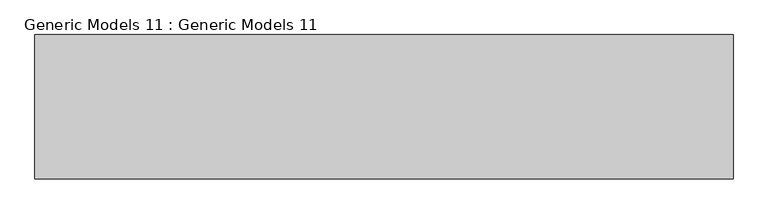
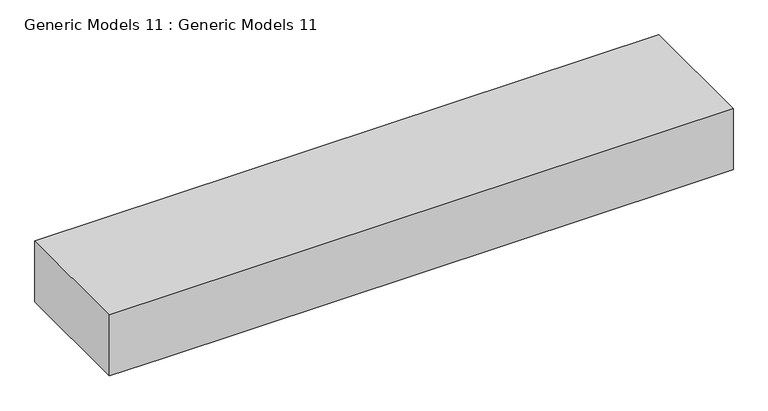
"""IFC4 building model written with IfcOpenShell, lengths in millimetres: proxy geometry, Generic Models 11 : Generic Models 11."""

from ifc_helpers import new_model, si_unit, frame, origin, place, context, project, spatial, polyline, outline, extrude, source, transform, mapped, element, save


def generic_models_11_generic_models_11_d301a5e8(model_context):
    return source(origin(), model_context, "Body", "SweptSolid", [
        extrude(outline(polyline([(17373.6, 2479.7847416), (17373.6, 3698.9847416), (17373.6, 3825.9847416), (17526.0, 3825.9847416), (17526.0, 2352.7847416), (17373.6, 2352.7847416), (17373.6, 2479.7847416)])), frame((0.0, 13271.2309003, 0.0), z_axis=(0.0, 1.0, 0.0), x_axis=(0.0, 0.0, 1.0)), (0.0, 0.0, 1.0), 304.8),
    ])


if __name__ == "__main__":
    model = new_model("IFC4")
    model_context = context("Model", 3, world=origin())
    ifc_project = project(units=[si_unit("LENGTHUNIT", "METRE", prefix="MILLI")], contexts=[model_context])
    site = spatial("IfcSite", under=ifc_project)
    building = spatial("IfcBuilding", under=site)
    placement = place(None, origin())
    generic_models_11_generic_models_11_shape = generic_models_11_generic_models_11_d301a5e8(model_context)
    element("IfcBuildingElementProxy", 1, Name="Generic Models 11 : Generic Models 11", ObjectType="Generic Models 11 : Generic Models 11", at=placement, inside=building, context=model_context, shape_type="MappedRepresentation", body=[
        mapped(generic_models_11_generic_models_11_shape, transform((0.0, 0.0, 0.0), x_axis=(1.0, 0.0, 0.0), y_axis=(0.0, 1.0, 0.0), z_axis=(0.0, 0.0, 1.0))),
    ])
    save(model, "model.ifc")

# Revit data of these elements
# Element 1 (IfcBuildingElementProxy, "Generic Models 11 : Generic Models 11")
#   Materials on its faces: "white"
# Materials
#   "white": class "Generic", colour RGB 120 120 120, transparency 0, Cost = 0
